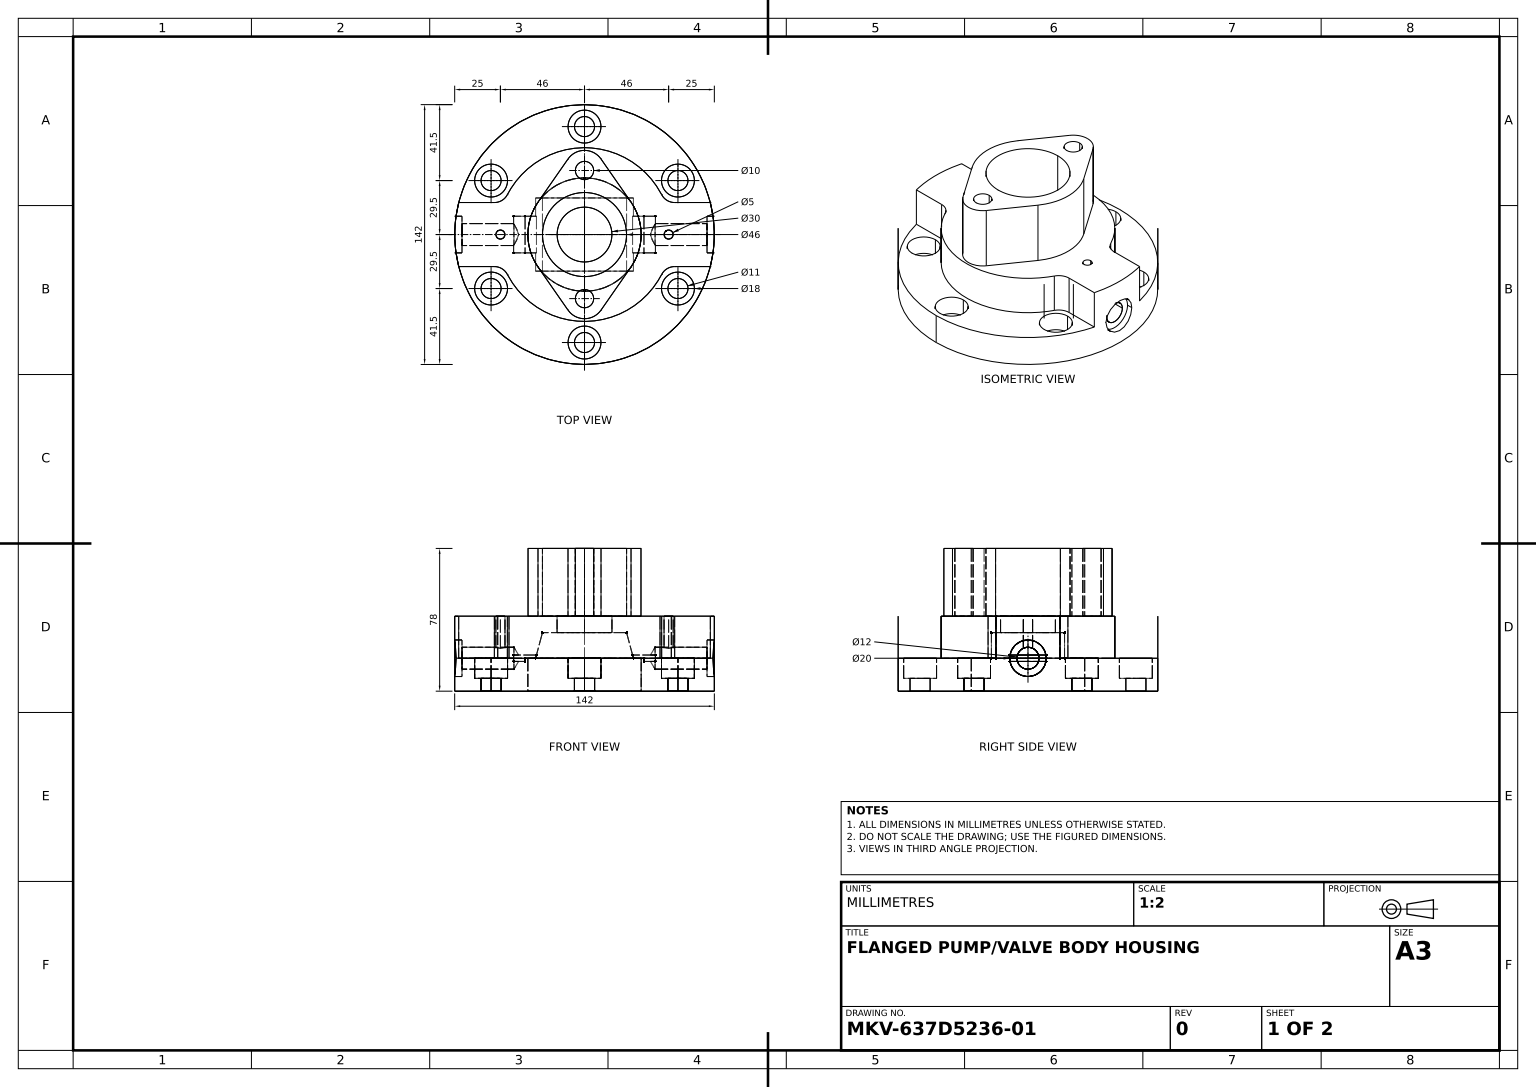
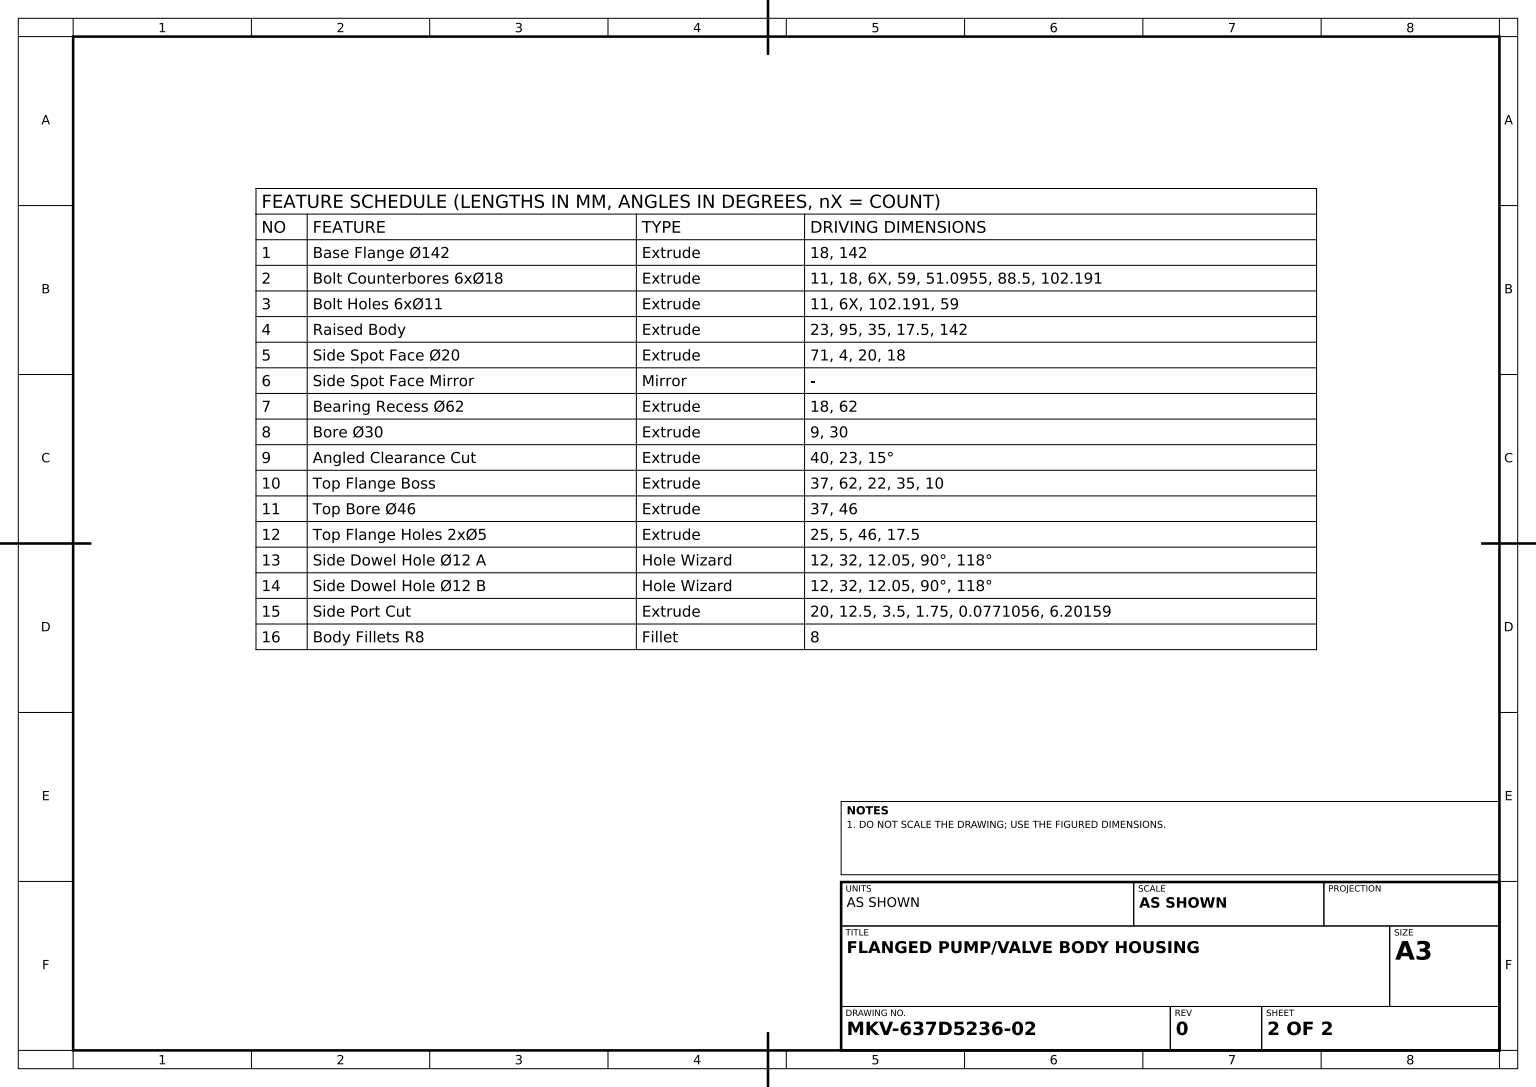
SolidWorks part; units mm, degrees
material "Plain Carbon Steel"
ref_plane "Front Plane" through (0, 0, 0) normal (0, 0, 1) x (1, 0, 0)
ref_plane "Top Plane" through (0, 0, 0) normal (0, 1, 0) x (1, 0, 0)
ref_plane "Right Plane" through (0, 0, 0) normal (1, 0, 0) x (0, 0, -1)
sketch "Base Flange Sketch" plane through (0, 0, 0) normal (0, 1, 0) x (1, 0, 0)
  circle A0 centre (0, 0) radius 71
  dimension "D1" = 142
extrude "Base Flange Ø142" add sketch "Base Flange Sketch" along normal blind 18
sketch "Counterbore Sketch" plane through (0, 18, 0) normal (0, 1, 0) x (1, 0, 0)
  circle A1 centre (0, 59) radius 9
  circle A2 centre (51.0955, 29.5) radius 9
  circle A3 centre (51.0955, -29.5) radius 9
  circle A4 centre (0, -59) radius 9
  circle A5 centre (-51.0955, -29.5) radius 9
  circle A6 centre (-51.0955, 29.5) radius 9
  dimension "D1" = 59
  dimension "D2" = 18
  dimension "D4" = 51.0955
  dimension "D5" = 88.5
  dimension "D6" = 102.191
  dimension "D3" = 6
extrude "Bolt Counterbores 6xØ18" cut sketch "Counterbore Sketch" against normal blind 11
sketch "Bolt Hole Sketch" plane through (0, 7, 0) normal (0, 1, 0) x (1, 0, 0)
  circle A0 centre (-51.0955, 29.5) radius 5.5
  circle A1 centre (0, 59) radius 5.5
  circle A2 centre (51.0955, 29.5) radius 5.5
  circle A3 centre (51.0955, -29.5) radius 5.5
  circle A4 centre (0, -59) radius 5.5
  circle A5 centre (-51.0955, -29.5) radius 5.5
  dimension "D1" = 11
  dimension "D3" = 102.191
  dimension "D4" = 59
  dimension "D2" = 6
extrude "Bolt Holes 6xØ11" cut sketch "Bolt Hole Sketch" against normal blind 11
sketch "Raised Body Sketch" plane through (0, 18, 0) normal (0, 1, 0) x (1, 0, 0)
  line L0 (0, -42.9) -> (0, 42.9) construction
  line L1 (-68.8095, 17.5) -> (-44.1588, 17.5)
  line L3 (-68.8095, -17.5) -> (-44.1588, -17.5)
  line L9 (68.8095, -17.5) -> (44.1588, -17.5)
  line L10 (68.8095, 17.5) -> (44.1588, 17.5)
  arc A0 (-44.1588, -17.5) -> (44.1588, -17.5) centre (0, 0) ccw
  arc A1 (68.8095, -17.5) -> (68.8095, 17.5) centre (0, 0) ccw
  arc A2 (44.1588, 17.5) -> (-44.1588, 17.5) centre (0, 0) ccw
  arc A3 (-68.8095, 17.5) -> (-68.8095, -17.5) centre (0, 0) ccw
  dimension "D1" = 95
  dimension "D4" = 142
  dimension "D2" = 35
  dimension "D3" = 17.5
extrude "Raised Body" add sketch "Raised Body Sketch" along normal blind 23
ref_plane "Plane1" through (71, 0, 0) normal (1, 0, 0) x (0, 0, -1)
sketch "Side Spot Face Sketch" plane through (71, 0, 0) normal (1, 0, 0) x (0, 0, -1)
  line L0 (-71, 0) -> (71, 0) construction
  line L1 (-71, 18) -> (-71, 0) construction
  circle A0 centre (0, 18) radius 10
  dimension "D1" = 20
  dimension "D2" = 18
  dimension "D3" = 71
extrude "Side Spot Face Ø20" cut sketch "Side Spot Face Sketch" against normal blind 4
mirror "Side Spot Face Mirror" about plane through (0, 0, 0) normal (1, 0, 0) of "Side Spot Face Ø20"
sketch "Bearing Recess Sketch" plane through (0, 0, 0) normal (0, -1, 0) x (1, 0, 0)
  circle A0 centre (0, 0) radius 31
  dimension "D1" = 62
extrude "Bearing Recess Ø62" cut sketch "Bearing Recess Sketch" against normal blind 18
sketch "Bore Ø30 Sketch" plane through (0, 41, 0) normal (0, 1, 0) x (1, 0, 0)
  circle A0 centre (0, 0) radius 15
  dimension "D1" = 30
extrude "Bore Ø30" cut sketch "Bore Ø30 Sketch" against normal blind 9
ref_plane "Plane4" through (0, 0, 0) normal (0, 0, 1) x (1, 0, 0)
sketch "Angled Cut Sketch" plane through (0, 0, 0) normal (0, 0, 1) x (1, 0, 0)
  line L0 (0, 32) -> (23, 32)
  line L1 (15, 32) -> (-15, 32) construction
  line L2 (23, 32) -> (26.7513, 18)
  line L3 (44.1588, 18) -> (-44.1588, 18) construction
  line L4 (0, 32) -> (-23, 32)
  line L5 (-23, 32) -> (-26.7513, 18)
  line L6 (-31, 18) -> (31, 18) construction
  line L7 (26.7513, 18) -> (-26.7513, 18)
  dimension "D1" = 23
  dimension "D2" = 23
  dimension "D3" = 15
  dimension "D4" = 15
extrude "Angled Clearance Cut" cut sketch "Angled Cut Sketch" against normal mid plane 40
sketch "Top Flange Boss Sketch" plane through (0, 41, 0) normal (0, 1, 0) x (1, 0, 0)
  line L0 (-9.0272, 41.2857) -> (-25.4402, 17.7143)
  line L1 (9.0272, 41.2857) -> (25.4402, 17.7143)
  line L2 (-9.0272, -41.2857) -> (-25.4402, -17.7143)
  line L3 (9.0272, -41.2857) -> (25.4402, -17.7143)
  arc A0 (-25.4402, 17.7143) -> (-25.4402, -17.7143) centre (0, 0) ccw
  arc A1 (9.0272, 41.2857) -> (-9.0272, 41.2857) centre (0, 35) ccw
  arc A2 (-9.0272, -41.2857) -> (9.0272, -41.2857) centre (0, -35) ccw
  circle A3 centre (0, 35) radius 5
  circle A4 centre (0, -35) radius 5
  arc A5 (25.4402, -17.7143) -> (25.4402, 17.7143) centre (0, 0) ccw
  dimension "D1" = 62
  dimension "D2" = 22
  dimension "D3" = 22
  dimension "D8" = 10
  dimension "D9" = 10
  dimension "D4" = 0
  dimension "D5" = 0
  dimension "D6" = 35
  dimension "D7" = 35
extrude "Top Flange Boss" add sketch "Top Flange Boss Sketch" along normal blind 37
sketch "Top Bore Sketch" plane through (0, 78, 0) normal (0, 1, 0) x (1, 0, 0)
  circle A0 centre (0, 0) radius 23
  dimension "D1" = 46
extrude "Top Bore Ø46" cut sketch "Top Bore Sketch" against normal blind 37
sketch "Top Flange Holes Sketch" plane through (0, 41, 0) normal (0, 1, 0) x (1, 0, 0)
  line L0 (68.8095, 17.5) -> (44.1588, 17.5) construction
  line L1 (-44.1588, 17.5) -> (-68.8095, 17.5) construction
  circle A0 centre (-46, 0) radius 2.5
  circle A1 centre (46, 0) radius 2.5
  dimension "D1" = 5
  dimension "D2" = 5
  dimension "D3" = 46
  dimension "D4" = 46
  dimension "D5" = 17.5
  dimension "D6" = 17.5
extrude "Top Flange Holes 2xØ5" cut sketch "Top Flange Holes Sketch" against normal blind 25
hole_wizard "Side Dowel Hole Ø12 A" positions "Sketch18" profile "Sketch19" hole size "Ø12.0" standard "ISO"
sketch "Sketch18" plane through (67, 0, 0) normal (1, 0, 0) x (0, 0, -1)
  point P0 (0, 18)
sketch "Sketch19" plane through (67, 18, 0) normal (0, 1, 0) x (0, 0, -1)
  line L0 (0, 0) -> (0, 32)
  line L1 (0, 32) -> (6, 28.3948)
  line L2 (6, 28.3948) -> (6, 0.025)
  line L3 (6, 0.025) -> (6.025, 0)
  line L5 (6.025, 0) -> (0, 0)
  line L6 (-6, 0.025) -> (-6.025, 0) construction
  line L10 (0, 32) -> (-6, 28.3948) construction
  line L11 (0, -6.35) -> (0, 107.95) construction
  dimension "Hole Dia." = 12
  dimension "Hole Depth" = 32
  dimension "Near C'Sink Dia." = 12.05
  dimension "Near C'Sink Angle" = 90
  dimension "Drill Angle" = 118
hole_wizard "Side Dowel Hole Ø12 B" positions "Sketch20" profile "Sketch21" hole size "Ø12.0" standard "ISO"
sketch "Sketch20" plane through (-67, 0, 0) normal (-1, 0, 0) x (0, 0, 1)
  point P0 (0, 18)
sketch "Sketch21" plane through (-67, 18, 0) normal (0, 1, 0) x (0, 0, 1)
  line L0 (0, 0) -> (0, 32)
  line L1 (0, 32) -> (6, 28.3948)
  line L2 (6, 28.3948) -> (6, 0.025)
  line L3 (6, 0.025) -> (6.025, 0)
  line L5 (6.025, 0) -> (0, 0)
  line L6 (-6, 0.025) -> (-6.025, 0) construction
  line L10 (0, 32) -> (-6, 28.3948) construction
  line L11 (0, -6.35) -> (0, 107.95) construction
  dimension "Hole Dia." = 12
  dimension "Hole Depth" = 32
  dimension "Near C'Sink Dia." = 12.05
  dimension "Near C'Sink Angle" = 90
  dimension "Drill Angle" = 118
ref_plane "Plane6" through (0, 0, 0) normal (0, 0, 1) x (1, 0, 0)
sketch "Side Port Sketch" plane through (0, 0, 0) normal (0, 0, 1) x (1, 0, 0)
  line L0 (26.2824, 19.75) -> (38.7824, 19.75)
  line L1 (26.7513, 18) -> (23, 32) construction
  line L2 (38.7824, 19.75) -> (38.7824, 16.25)
  line L3 (38.7824, 16.25) -> (32.5808, 16.25)
  line L6 (32.5037, 18) -> (26.7513, 18)
  line L7 (26.7513, 18) -> (26.2824, 19.75)
  line L8 (32.5037, 18) -> (32.5037, 16.25)
  line L9 (32.5037, 16.25) -> (32.5808, 16.25)
  line L10 (0, -42.9) -> (0, 42.9) construction
  line L11 (-32.5037, 16.25) -> (-32.5808, 16.25)
  line L12 (-32.5037, 18) -> (-32.5037, 16.25)
  line L13 (-32.5037, 18) -> (-26.7513, 18)
  line L14 (-26.7513, 18) -> (-26.2824, 19.75)
  line L15 (-26.2824, 19.75) -> (-38.7824, 19.75)
  line L16 (-38.7824, 19.75) -> (-38.7824, 16.25)
  line L17 (-38.7824, 16.25) -> (-32.5808, 16.25)
  dimension "D1" = 12.5
  dimension "D2" = 3.5
  dimension "D3" = 1.75
  dimension "D4" = 0.0771
  dimension "D5" = 1.75
  dimension "D6" = 6.2016
extrude "Side Port Cut" cut sketch "Side Port Sketch" against normal mid plane 20
fillet "Body Fillets R8" radius 8 4 edges at (-44.1588, 29.5, -17.5) (-44.1588, 29.5, 17.5) (44.1588, 29.5, 17.5) (44.1588, 29.5, -17.5)
